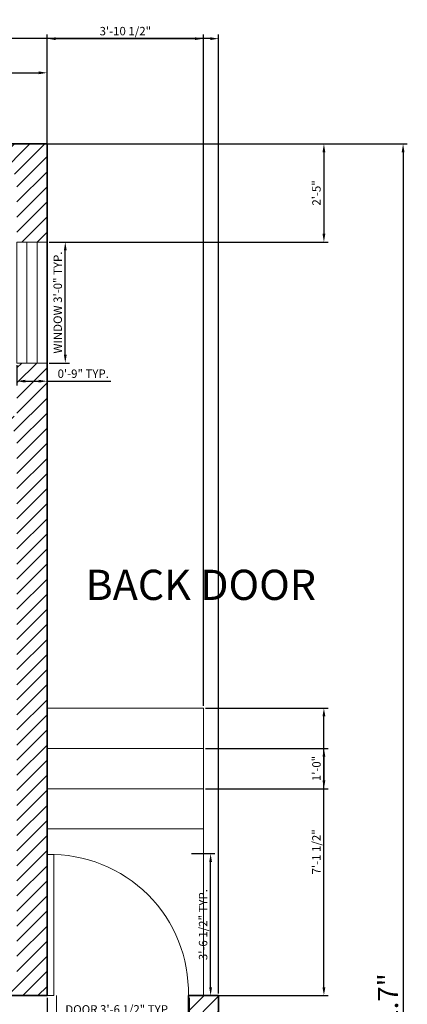
# Model space of a CAD drawing. Units: inches. Extents: x 4740 to 5323, y 7115 to 7713.
# Tile 6 of 6: x 5208 to 5323, y 7420 to 7713. Entities that reach past the tile are written whole.
import ezdxf

# ---------------------------------------------------------------- set-up
doc = ezdxf.new("R2010")
doc.units = ezdxf.units.IN
for name, color, linetype, lineweight in [('A-ANNO-DIMS', 2, 'Continuous', 18), ('A-ANNO-TEXT', 7, 'Continuous', 25), ('A-DOOR', 4, 'Continuous', 18), ('A-FLOR-STRS', 7, 'Continuous', 18), ('A-GLAZ', 242, 'Continuous', 18), ('A-WALL', 7, 'Continuous', 35)]:
    doc.layers.add(name, color=color, linetype=linetype, lineweight=lineweight)
doc.layers.add('A-WALL-PATT', color=152, linetype='Continuous', lineweight=13, true_color=0x2776bb)
doc.styles.get("Standard").update_dxf_attribs({"font": 'arial.ttf'})
doc.dimstyles.new('ISO-25', dxfattribs={"dimtxt": 2.5, "dimasz": 2.5, "dimexe": 1.25, "dimexo": 0.625, "dimtad": 1, "dimlunit": 3, "dimtxsty": 'Standard', "dimcen": 2.5, "dimadec": 0, "dimazin": 0, "dimtfac": 1, "dimtmove": 0, "dimatfit": 3, "dimfxl": 1, "dimarcsym": 0})

# ---------------------------------------------------------------- blocks, each defined once
blk = doc.blocks.new('*D35')
at = {"layer": 'A-ANNO-DIMS', "color": 0, "lineweight": -2, "transparency": 16777216}
for p, q in [((4776.46, 7632.98), (4776.46, 7698.25)), ((5215.96, 7629.25), (5215.96, 7698.25)), ((4778.96, 7697), (5213.46, 7697))]:
    blk.add_line(p, q, dxfattribs=at)
at = {"layer": 'A-ANNO-DIMS', "color": 0, "transparency": 16777216}
for points in [[(4778.96, 7697.42), (4778.96, 7696.58), (4776.46, 7697)], [(5213.46, 7697.42), (5213.46, 7696.58), (5215.96, 7697)]]:
    blk.add_solid(points, dxfattribs=at)
at = {"layer": 'Defpoints', "color": 0, "transparency": 16777216}
for p in [(5215.96, 7697), (4776.46, 7632.36), (5215.96, 7628.62)]:
    blk.add_point(p, dxfattribs=at)
at = {"layer": 'A-ANNO-DIMS', "color": 0, "transparency": 16777216, "insert": (4996.21, 7700.69), "char_height": 6, "attachment_point": 5}
blk.add_mtext('36\'-7.5"', dxfattribs=at)
blk = doc.blocks.new('*D36')
at = {"layer": 'A-ANNO-DIMS', "color": 0, "lineweight": -2, "transparency": 16777216}
for p, q in [((5078.58, 7675.86), (5323.05, 7675.86)), ((5321.8, 7673.36), (5321.8, 7150.66)), ((5077.56, 7148.16), (5323.05, 7148.16))]:
    blk.add_line(p, q, dxfattribs=at)
at = {"layer": 'A-ANNO-DIMS', "color": 0, "transparency": 16777216}
for points in [[(5321.38, 7673.36), (5322.22, 7673.36), (5321.8, 7675.86)], [(5321.38, 7150.66), (5322.22, 7150.66), (5321.8, 7148.16)]]:
    blk.add_solid(points, dxfattribs=at)
at = {"layer": 'Defpoints', "color": 0, "transparency": 16777216}
for p in [(5077.96, 7675.86), (5076.93, 7148.16), (5321.8, 7148.16)]:
    blk.add_point(p, dxfattribs=at)
at = {"layer": 'A-ANNO-DIMS', "color": 0, "transparency": 16777216, "insert": (5318.11, 7412.01), "char_height": 6, "attachment_point": 5, "rotation": 90}
blk.add_mtext('43\'-11.7"', dxfattribs=at)
blk = doc.blocks.new('WIN-36IN')
for p, q in [((0, 36), (9, 36)), ((0, 36), (0, 0)), ((3, 36), (3, 0)), ((6, 36), (6, 0)), ((9, 0), (9, 36)), ((0, 0), (9, 0))]:
    blk.add_line(p, q)
blk = doc.blocks.new('DOOR-SWING-42IN')
for p, q in [((0, 0), (0, 42)), ((0, 42), (2, 42)), ((2, 42), (2, 0)), ((2, 0), (0, 0))]:
    blk.add_line(p, q)
blk.add_arc((1, 1), 41.01, 358.6028, 91.3972)
blk = doc.blocks.new('*D46')
at = {"layer": 'A-ANNO-DIMS', "color": 0, "lineweight": -2, "transparency": 16777216}
for p, q in [((5216.58, 7646.62), (5222.61, 7646.62)), ((5221.36, 7613.12), (5221.36, 7644.12)), ((5216.58, 7610.62), (5222.61, 7610.62))]:
    blk.add_line(p, q, dxfattribs=at)
at = {"layer": 'A-ANNO-DIMS', "color": 0, "transparency": 16777216}
for points in [[(5220.94, 7644.12), (5221.78, 7644.12), (5221.36, 7646.62)], [(5220.94, 7613.12), (5221.78, 7613.12), (5221.36, 7610.62)]]:
    blk.add_solid(points, dxfattribs=at)
at = {"layer": 'Defpoints', "color": 0, "transparency": 16777216}
for p in [(5215.96, 7646.62), (5221.36, 7646.62), (5215.96, 7610.62)]:
    blk.add_point(p, dxfattribs=at)
at = {"layer": 'A-ANNO-DIMS', "color": 0, "transparency": 16777216, "insert": (5219.44, 7628.62), "char_height": 2.5, "attachment_point": 5, "rotation": 90}
blk.add_mtext('WINDOW 3\'-0" TYP.', dxfattribs=at)
blk = doc.blocks.new('*D47')
at = {"layer": 'A-ANNO-DIMS', "color": 0, "lineweight": -2, "transparency": 16777216}
for p, q in [((5206.96, 7610), (5206.96, 7603.97)), ((5215.96, 7610), (5215.96, 7603.97)), ((5209.46, 7605.22), (5213.46, 7605.22)), ((5215.96, 7605.22), (5234.95, 7605.22))]:
    blk.add_line(p, q, dxfattribs=at)
at = {"layer": 'A-ANNO-DIMS', "color": 0, "transparency": 16777216}
for points in [[(5209.46, 7605.64), (5209.46, 7604.81), (5206.96, 7605.22)], [(5213.46, 7605.64), (5213.46, 7604.81), (5215.96, 7605.22)]]:
    blk.add_solid(points, dxfattribs=at)
at = {"layer": 'Defpoints', "color": 0, "transparency": 16777216}
for p in [(5206.96, 7610.62), (5215.96, 7610.62), (5215.96, 7605.22)]:
    blk.add_point(p, dxfattribs=at)
at = {"layer": 'A-ANNO-DIMS', "color": 0, "transparency": 16777216, "insert": (5226.7, 7607.13), "char_height": 2.5, "attachment_point": 5}
blk.add_mtext('0\'-9" TYP.', dxfattribs=at)
blk = doc.blocks.new('*D58')
at = {"layer": 'A-ANNO-DIMS', "color": 0, "lineweight": -2, "transparency": 16777216}
for p, q in [((5215.96, 7421.73), (5215.96, 7414.77)), ((5258.23, 7421.73), (5258.23, 7414.77)), ((5218.46, 7416.02), (5255.73, 7416.02))]:
    blk.add_line(p, q, dxfattribs=at)
at = {"layer": 'A-ANNO-DIMS', "color": 0, "transparency": 16777216}
for points in [[(5218.46, 7416.43), (5218.46, 7415.6), (5215.96, 7416.02)], [(5255.73, 7416.43), (5255.73, 7415.6), (5258.23, 7416.02)]]:
    blk.add_solid(points, dxfattribs=at)
at = {"layer": 'Defpoints', "color": 0, "transparency": 16777216}
for p in [(5215.96, 7422.36), (5258.23, 7422.36), (5258.23, 7416.02)]:
    blk.add_point(p, dxfattribs=at)
at = {"layer": 'A-ANNO-DIMS', "color": 0, "transparency": 16777216, "insert": (5237.1, 7417.94), "char_height": 2.5, "attachment_point": 5}
blk.add_mtext('DOOR 3\'-6 1/2" TYP.', dxfattribs=at)
blk = doc.blocks.new('*D59')
at = {"layer": 'A-ANNO-DIMS', "color": 0, "lineweight": -2, "transparency": 16777216}
for p, q in [((5258.86, 7464.63), (5265.82, 7464.63)), ((5264.57, 7424.86), (5264.57, 7462.13)), ((5258.86, 7422.36), (5265.82, 7422.36))]:
    blk.add_line(p, q, dxfattribs=at)
at = {"layer": 'A-ANNO-DIMS', "color": 0, "transparency": 16777216}
for points in [[(5264.16, 7462.13), (5264.99, 7462.13), (5264.57, 7464.63)], [(5264.16, 7424.86), (5264.99, 7424.86), (5264.57, 7422.36)]]:
    blk.add_solid(points, dxfattribs=at)
at = {"layer": 'Defpoints', "color": 0, "transparency": 16777216}
for p in [(5258.23, 7464.63), (5264.57, 7464.63), (5258.23, 7422.36)]:
    blk.add_point(p, dxfattribs=at)
at = {"layer": 'A-ANNO-DIMS', "color": 0, "transparency": 16777216, "insert": (5262.66, 7443.49), "char_height": 2.5, "attachment_point": 5, "rotation": 90}
blk.add_mtext('3\'-6 1/2" TYP.', dxfattribs=at)
blk = doc.blocks.new('*D75')
at = {"layer": 'A-ANNO-DIMS', "color": 0, "lineweight": -2, "transparency": 16777216}
for p, q in [((5216.58, 7675.86), (5299.51, 7675.86)), ((5298.26, 7673.36), (5298.26, 7649.12)), ((5216.58, 7646.62), (5299.51, 7646.62))]:
    blk.add_line(p, q, dxfattribs=at)
at = {"layer": 'A-ANNO-DIMS', "color": 0, "transparency": 16777216}
for points in [[(5297.84, 7673.36), (5298.68, 7673.36), (5298.26, 7675.86)], [(5297.84, 7649.12), (5298.68, 7649.12), (5298.26, 7646.62)]]:
    blk.add_solid(points, dxfattribs=at)
at = {"layer": 'Defpoints', "color": 0, "transparency": 16777216}
for p in [(5215.96, 7675.86), (5215.96, 7646.62), (5298.26, 7646.62)]:
    blk.add_point(p, dxfattribs=at)
at = {"layer": 'A-ANNO-DIMS', "color": 0, "transparency": 16777216, "insert": (5296.36, 7661.24), "char_height": 2.5, "attachment_point": 5, "rotation": 90}
blk.add_mtext('2\'-5"', dxfattribs=at)
blk = doc.blocks.new('*D81')
at = {"layer": 'A-ANNO-DIMS', "color": 0, "lineweight": -2, "transparency": 16777216}
for p, q in [((4776.46, 7632.98), (4776.46, 7708.41)), ((5264.46, 7707.16), (4778.96, 7707.16)), ((5266.96, 7422.98), (5266.96, 7708.41))]:
    blk.add_line(p, q, dxfattribs=at)
at = {"layer": 'A-ANNO-DIMS', "color": 0, "transparency": 16777216}
for points in [[(4778.96, 7707.57), (4778.96, 7706.74), (4776.46, 7707.16)], [(5264.46, 7707.57), (5264.46, 7706.74), (5266.96, 7707.16)]]:
    blk.add_solid(points, dxfattribs=at)
at = {"layer": 'Defpoints', "color": 0, "transparency": 16777216}
for p in [(4776.46, 7707.16), (4776.46, 7632.36), (5266.96, 7422.36)]:
    blk.add_point(p, dxfattribs=at)
at = {"layer": 'A-ANNO-DIMS', "color": 0, "transparency": 16777216, "insert": (5021.71, 7709.07), "char_height": 2.5, "attachment_point": 5}
blk.add_mtext('40\'-10 1/2"', dxfattribs=at)
blk = doc.blocks.new('*D83')
at = {"layer": 'A-ANNO-DIMS', "color": 0, "lineweight": -2, "transparency": 16777216}
for p, q in [((5215.96, 7508.58), (5215.96, 7708.41)), ((5218.46, 7707.16), (5259.96, 7707.16)), ((5262.46, 7508.58), (5262.46, 7708.41))]:
    blk.add_line(p, q, dxfattribs=at)
at = {"layer": 'A-ANNO-DIMS', "color": 0, "transparency": 16777216}
for points in [[(5218.46, 7707.57), (5218.46, 7706.74), (5215.96, 7707.16)], [(5259.96, 7707.57), (5259.96, 7706.74), (5262.46, 7707.16)]]:
    blk.add_solid(points, dxfattribs=at)
at = {"layer": 'Defpoints', "color": 0, "transparency": 16777216}
for p in [(5262.46, 7707.16), (5215.96, 7507.95), (5262.46, 7507.95)]:
    blk.add_point(p, dxfattribs=at)
at = {"layer": 'A-ANNO-DIMS', "color": 0, "transparency": 16777216, "insert": (5239.21, 7709.08), "char_height": 2.5, "attachment_point": 5}
blk.add_mtext('3\'-10 1/2"', dxfattribs=at)
blk = doc.blocks.new('*D84')
at = {"layer": 'A-ANNO-DIMS', "color": 0, "lineweight": -2, "transparency": 16777216}
for p, q in [((5263.08, 7507.95), (5299.51, 7507.95)), ((5298.26, 7424.86), (5298.26, 7505.45)), ((5263.08, 7422.36), (5299.51, 7422.36))]:
    blk.add_line(p, q, dxfattribs=at)
at = {"layer": 'A-ANNO-DIMS', "color": 0, "transparency": 16777216}
for points in [[(5297.84, 7505.45), (5298.68, 7505.45), (5298.26, 7507.95)], [(5297.84, 7424.86), (5298.68, 7424.86), (5298.26, 7422.36)]]:
    blk.add_solid(points, dxfattribs=at)
at = {"layer": 'Defpoints', "color": 0, "transparency": 16777216}
for p in [(5262.46, 7507.95), (5298.26, 7507.95), (5262.46, 7422.36)]:
    blk.add_point(p, dxfattribs=at)
at = {"layer": 'A-ANNO-DIMS', "color": 0, "transparency": 16777216, "insert": (5296.34, 7465.15), "char_height": 2.5, "attachment_point": 5, "rotation": 90}
blk.add_mtext('7\'-1 1/2"', dxfattribs=at)
blk = doc.blocks.new('*D85')
at = {"layer": 'A-ANNO-DIMS', "color": 0, "lineweight": -2, "transparency": 16777216}
for p, q in [((5263.08, 7495.95), (5299.51, 7495.95)), ((5298.26, 7493.45), (5298.26, 7486.45)), ((5263.08, 7483.95), (5299.51, 7483.95))]:
    blk.add_line(p, q, dxfattribs=at)
at = {"layer": 'A-ANNO-DIMS', "color": 0, "transparency": 16777216}
for points in [[(5297.84, 7493.45), (5298.68, 7493.45), (5298.26, 7495.95)], [(5297.84, 7486.45), (5298.68, 7486.45), (5298.26, 7483.95)]]:
    blk.add_solid(points, dxfattribs=at)
at = {"layer": 'Defpoints', "color": 0, "transparency": 16777216}
for p in [(5262.46, 7495.95), (5262.46, 7483.95), (5298.26, 7483.95)]:
    blk.add_point(p, dxfattribs=at)
at = {"layer": 'A-ANNO-DIMS', "color": 0, "transparency": 16777216, "insert": (5296.36, 7489.95), "char_height": 2.5, "attachment_point": 5, "rotation": 90}
blk.add_mtext('1\'-0"', dxfattribs=at)

msp = doc.modelspace()

# ---------------------------------------------------------------- hatches: boundary and pattern name
at = {"layer": 'A-WALL-PATT'}
h = msp.add_hatch(dxfattribs=at)
h.set_pattern_fill('ANSI31', color=256)
h.paths.add_polyline_path([(4925.343, 7632.357), (4776.459, 7632.357), (4776.459, 7486.448), (4785.459, 7486.448), (4785.459, 7522.857), (4959.459, 7522.857), (4959.459, 7527.357), (4785.459, 7527.357), (4785.459, 7623.357), (4833.459, 7623.357), (4925.343, 7623.357)])
h.paths.add_polyline_path([(5010.258, 7599.357), (5004.258, 7599.357), (4986.459, 7599.357), (4986.459, 7623.357), (4986.459, 7632.357), (4977.459, 7632.357), (4949.343, 7632.357), (4949.343, 7623.357), (4977.459, 7623.357), (4977.459, 7599.357), (4977.459, 7594.857), (4977.459, 7590.357), (4977.459, 7524.857, -0.0293864), (4977.459, 7522.857), (4977.459, 7426.857), (4977.459, 7422.357), (4977.459, 7419.778), (4981.959, 7419.778), (4981.959, 7422.357), (5041.959, 7422.357), (5041.959, 7479.357), (5037.459, 7479.357), (5037.459, 7426.857), (4981.959, 7426.857), (4981.959, 7590.357), (5010.258, 7590.357)])
h.paths.add_polyline_path([(5086.959, 7666.857), (5206.959, 7666.857), (5206.959, 7646.624), (5215.959, 7646.624), (5215.959, 7675.857), (5077.959, 7675.857), (5077.959, 7599.357), (5046.258, 7599.357), (5046.258, 7590.357), (5082.459, 7590.357), (5082.459, 7474.857, -0.0106371), (5084.459, 7474.857), (5086.959, 7474.857)])
h.paths.add_polyline_path([(5215.959, 7610.624), (5206.959, 7610.624), (5206.959, 7594.857), (5104.959, 7594.857), (5104.959, 7592.357, -0.0293864), (5104.959, 7590.357), (5206.959, 7590.357), (5206.959, 7426.857), (5104.959, 7426.857), (5082.459, 7426.857), (5082.459, 7422.357), (5104.959, 7422.357), (5215.959, 7422.357), (5215.959, 7464.357), (5215.959, 7506.357)])
h.paths.add_polyline_path([(4881.459, 7375.857), (4977.459, 7375.857), (4977.459, 7296.657), (4981.959, 7296.657), (4981.959, 7384.857), (4951.959, 7384.857), (4785.459, 7384.857), (4785.459, 7438.448), (4776.459, 7438.448), (4776.459, 7375.857), (4872.459, 7375.857), (4872.459, 7337.044), (4881.459, 7337.044)])
h.paths.add_polyline_path([(4881.459, 7313.044), (4872.459, 7313.044), (4872.459, 7148.157), (4916.568, 7148.157), (4916.568, 7157.157), (4881.459, 7157.157), (4881.459, 7269.357), (4981.959, 7269.357), (4981.959, 7273.857), (4963.959, 7273.857), (4881.459, 7273.857)])
h.paths.add_polyline_path([(5029.959, 7296.657), (5116.509, 7296.657), (5116.509, 7299.157, -0.0121933), (5116.509, 7301.157), (5025.459, 7301.157), (5025.459, 7157.157), (4964.568, 7157.157), (4964.568, 7148.157), (5076.933, 7148.157), (5076.933, 7157.157), (5029.959, 7157.157)])
h.paths.add_polyline_path([(5182.959, 7203.442), (5173.959, 7203.442), (5173.959, 7157.157), (5124.933, 7157.157), (5124.933, 7148.157), (5182.959, 7148.157)])
h.paths.add_polyline_path([(5266.959, 7353.764), (5257.959, 7353.764), (5257.959, 7301.157), (5182.959, 7301.157), (5158.509, 7301.157), (5158.509, 7296.657), (5173.959, 7296.657), (5173.959, 7263.442), (5182.959, 7263.442), (5182.959, 7292.157), (5266.959, 7292.157)])
h.paths.add_polyline_path([(5266.959, 7422.357), (5257.959, 7422.357), (5257.959, 7377.764), (5266.959, 7377.764)])

# ---------------------------------------------------------------- linework, layer by layer
at = {"layer": 'A-FLOR-STRS'}
for p, q in [((5262.459, 7507.951), (5215.959, 7507.951)), ((5262.459, 7422.357), (5262.459, 7507.951)), ((5262.459, 7495.951), (5215.959, 7495.951)), ((5262.459, 7483.951), (5215.959, 7483.951)), ((5262.459, 7471.951), (5215.959, 7471.951)), ((5218.734, 7301.157), (5218.734, 7422.357))]:
    msp.add_line(p, q, dxfattribs=at)
at = {"layer": 'A-WALL'}
for p, q in [((5077.959, 7675.857), (5215.959, 7675.857)), ((5215.959, 7675.857), (5215.959, 7422.357)), ((5215.959, 7464.357), (5215.959, 7506.357)), ((5215.959, 7422.357), (5215.959, 7464.357)), ((5104.959, 7422.357), (5215.959, 7422.357)), ((5257.959, 7422.357), (5257.959, 7301.157)), ((5257.959, 7422.357), (5266.959, 7422.357)), ((5266.959, 7422.357), (5266.959, 7292.157))]:
    msp.add_line(p, q, dxfattribs=at)

# ---------------------------------------------------------------- block references
at = {"layer": 'A-DOOR'}
msp.add_blockref('DOOR-SWING-42IN', (5215.959, 7422.357), dxfattribs=at)
at = {"layer": 'A-GLAZ'}
msp.add_blockref('WIN-36IN', (5206.959, 7610.624), dxfattribs=at)

# ---------------------------------------------------------------- texts
at = {"layer": 'A-ANNO-TEXT', "insert": (5227.4, 7549.107), "char_height": 9, "attachment_point": 1}
msp.add_mtext_dynamic_manual_height_columns('\\pxt8;{BACK DOOR}', width=75.84022, gutter_width=12.5, heights=[0], dxfattribs=at)

# ---------------------------------------------------------------- dimensions: what is measured, and where the dimension line sits
at = {"layer": 'A-ANNO-DIMS'}
for base, p1, p2, override, picture, middle in [((4776.459, 7707.157), (5266.959, 7422.357), (4776.459, 7632.357), {"dimdec": 1, "dimlfac": 1, "dimrnd": 0, "dimzin": 1, "dimdsep": 46, "dimlunit": 4, "dimfrac": 2}, '*D81', (5021.709, 7709.074)), ((5262.459, 7707.157), (5215.959, 7507.951), (5262.459, 7507.951), {"dimdec": 1, "dimlfac": 1, "dimrnd": 0, "dimzin": 1, "dimdsep": 46, "dimlunit": 4, "dimfrac": 2}, '*D83', (5239.209, 7709.075)), ((5215.959, 7697.001), (4776.459, 7632.357), (5215.959, 7628.624), {"dimtxt": 6, "dimclrd": 0, "dimclre": 0, "dimclrt": 0}, '*D35', (4996.209, 7700.692))]:
    dim = msp.add_linear_dim(base=base, p1=p1, p2=p2, dimstyle='ISO-25', override=override, dxfattribs=at)
    dim.commit()
    dim.dimension.update_dxf_attribs({"geometry": picture, "text_midpoint": middle})
for base, p1, p2, override, picture, middle in [((5321.801, 7148.157), (5077.959, 7675.857), (5076.933, 7148.157), {"dimtxt": 6, "dimclrd": 0, "dimclre": 0, "dimclrt": 0}, '*D36', (5318.111, 7412.007)), ((5298.259, 7646.624), (5215.959, 7675.857), (5215.959, 7646.624), {"dimdec": 1, "dimlfac": 1, "dimrnd": 0, "dimzin": 1, "dimdsep": 46, "dimlunit": 4, "dimfrac": 2}, '*D75', (5296.358, 7661.24)), ((5298.259, 7507.951), (5262.459, 7422.357), (5262.459, 7507.951), {"dimdec": 1, "dimlfac": 1, "dimrnd": 0, "dimzin": 1, "dimdsep": 46, "dimlunit": 4, "dimfrac": 2}, '*D84', (5296.342, 7465.154)), ((5298.259, 7483.951), (5262.459, 7495.951), (5262.459, 7483.951), {"dimdec": 1, "dimlfac": 1, "dimrnd": 0, "dimzin": 1, "dimdsep": 46, "dimlunit": 4, "dimfrac": 2}, '*D85', (5296.358, 7489.951))]:
    dim = msp.add_linear_dim(base=base, p1=p1, p2=p2, angle=90, dimstyle='ISO-25', override=override, dxfattribs=at)
    dim.commit()
    dim.dimension.update_dxf_attribs({"geometry": picture, "text_midpoint": middle})
for base, p1, p2, text, picture, middle in [((5221.359, 7646.624), (5215.959, 7610.624), (5215.959, 7646.624), 'WINDOW <> TYP.', '*D46', (5219.44, 7628.624)), ((5264.574, 7464.63), (5258.233, 7422.357), (5258.233, 7464.63), '<> TYP.', '*D59', (5262.655, 7443.494))]:
    dim = msp.add_linear_dim(base=base, p1=p1, p2=p2, angle=90, text=text, dimstyle='ISO-25', override={"dimdec": 1, "dimlfac": 1, "dimrnd": 0, "dimzin": 1, "dimdsep": 46, "dimlunit": 4, "dimfrac": 2}, dxfattribs=at)
    dim.commit()
    dim.dimension.update_dxf_attribs({"geometry": picture, "text_midpoint": middle})
for base, p1, p2, text, picture, middle in [((5215.959, 7605.224), (5206.959, 7610.624), (5215.959, 7610.624), '<> TYP.', '*D47', (5226.704, 7607.125)), ((5258.233, 7416.016), (5215.959, 7422.357), (5258.233, 7422.357), 'DOOR <> TYP.', '*D58', (5237.096, 7417.935))]:
    dim = msp.add_linear_dim(base=base, p1=p1, p2=p2, text=text, dimstyle='ISO-25', override={"dimdec": 1, "dimlfac": 1, "dimrnd": 0, "dimzin": 1, "dimdsep": 46, "dimlunit": 4, "dimfrac": 2}, dxfattribs=at)
    dim.commit()
    dim.dimension.update_dxf_attribs({"geometry": picture, "text_midpoint": middle})

doc.saveas('drawing.dxf')
